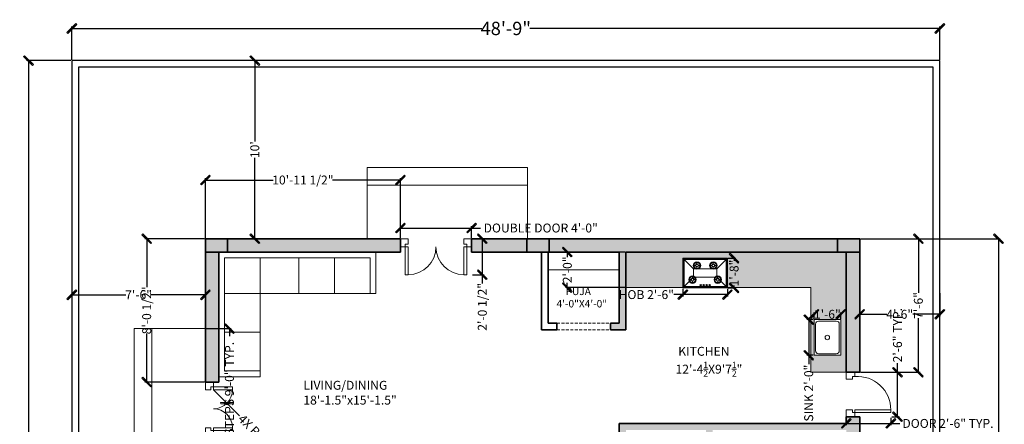
# Model space of a CAD drawing. Units: inches. Extents: x 1018 to 2596, y 723 to 1501.
# Tile 5 of 6: x 1018 to 1681, y 1229 to 1501. Entities that reach past the tile are written whole.
import ezdxf

# ---------------------------------------------------------------- set-up
doc = ezdxf.new("R2010")
doc.units = ezdxf.units.IN
doc.linetypes.add('DASHED2', pattern=[0.375, 0.25, -0.125])
doc.layers.get('Defpoints').update_dxf_attribs({"lineweight": 0})
for name, color, linetype, lineweight in [('A-ANNO-DIMS', 2, 'Continuous', 13), ('A-AREA-IDEN', 7, 'Continuous', 18), ('A-COLS', 7, 'Continuous', 35), ('A-DOOR', 4, 'Continuous', 18), ('A-EQPM', 8, 'Continuous', 18), ('A-FLOR-CASE', 8, 'Continuous', 18), ('A-FLOR-CASE-PATT', 9, 'Continuous', 9), ('A-FLOR-FIXT', 9, 'Continuous', 18), ('A-FLOR-STRS', 7, 'Continuous', 18), ('A-FURN', 8, 'Continuous', 13), ('A-WALL', 7, 'Continuous', 35), ('A-WALL-OVHD', 7, 'DASHED2', 13), ('C-PROP', 7, 'Continuous', 25)]:
    doc.layers.add(name, color=color, linetype=linetype, lineweight=lineweight)
doc.layers.add('A-WALL-PATT', color=9, linetype='Continuous', lineweight=9, true_color=0xc7c8ca)
doc.styles.get("Standard").update_dxf_attribs({"font": 'arial.ttf'})
doc.dimstyles.new('saketh', dxfattribs={"dimtxt": 6, "dimasz": 6, "dimexe": 1.25, "dimexo": 0.625, "dimtad": 0, "dimdec": 1, "dimlunit": 4, "dimtxsty": 'Standard', "dimblk": 'ARCHTICK', "dimcen": 2.5, "dimclrd": 256, "dimclre": 1, "dimadec": 0, "dimazin": 0, "dimtfac": 1, "dimtdec": 1, "dimtmove": 0, "dimatfit": 3, "dimldrblk": 'ARCHTICK', "dimfxl": 1, "dimtolj": 1, "dimarcsym": 0})

# ---------------------------------------------------------------- blocks, each defined once
blk = doc.blocks.new('4 feet double door')
at = {"layer": 'A-DOOR'}
for points in [[(3.28, 5.56), (3.28, 24.28), (5.25, 24.28), (5.25, 5.56)], [(44.72, 5.56), (44.72, 24.28), (42.75, 24.28), (42.75, 5.56)], [(3.28, 5.56), (0, 5.56), (0, 0), (5.25, 0), (5.25, 3.59), (3.28, 3.59)], [(44.72, 5.56), (48, 5.56), (48, 0), (42.75, 0), (42.75, 3.59), (44.72, 3.59)]]:
    blk.add_lwpolyline(points, close=True, dxfattribs=at)
at = {"layer": 'A-DOOR', "ltscale": 0.1}
for centre, start, end in [((5.25, 5.53), 0.09557, 90), ((42.75, 5.53), 90, 179.90443)]:
    blk.add_arc(centre, 18.75, start, end, dxfattribs=at)
blk = doc.blocks.new('3 1')
at = {"layer": 'A-DOOR'}
for points in [[(-32.72, 5.56), (-32.72, 18.28), (-30.75, 18.28), (-30.75, 5.56)], [(-3.28, 5.56), (-3.28, 18.28), (-5.25, 18.28), (-5.25, 5.56)], [(-32.72, 5.56), (-36, 5.56), (-36, 0), (-30.75, 0), (-30.75, 3.59), (-32.72, 3.59)], [(-5.25, 3.59), (-5.25, 0), (0, 0), (0, 5.56), (-3.28, 5.56), (-3.28, 3.59)]]:
    blk.add_lwpolyline(points, close=True, dxfattribs=at)
at = {"layer": 'A-DOOR', "ltscale": 0.1}
for centre, start, end in [((-30.75, 5.53), 0.1406, 90), ((-5.25, 5.53), 90, 179.8594)]:
    blk.add_arc(centre, 12.75, start, end, dxfattribs=at)
blk = doc.blocks.new('2 feet 6 inch door')
at = {"layer": 'A-DOOR'}
for points in [[(2.92, 5.83), (2.92, 30), (4.67, 30), (4.67, 5.83)], [(2.92, 4.08), (4.67, 4.08), (4.67, 0), (0, 0), (0, 5.83), (2.92, 5.83)], [(27.08, 5.83), (27.08, 4.08), (25.33, 4.08), (25.33, 0), (30, 0), (30, 5.83)]]:
    blk.add_lwpolyline(points, close=True, dxfattribs=at)
at = {"layer": 'A-DOOR', "ltscale": 0.1}
blk.add_arc((4.67, 7.52), 22.48, 355.69715, 90, dxfattribs=at)
blk = doc.blocks.new('_ArchTick')
for p, q in [((0.45, 0.55), (-0.55, -0.45)), ((-0.45, -0.55), (0.55, 0.45)), ((0.55, 0.45), (0.45, 0.55)), ((-0.55, -0.45), (-0.45, -0.55))]:
    blk.add_line(p, q)
mesh = blk.add_polyface()
corners = [(-0.45, -0.55), (0.45, 0.55), (-0.55, -0.45), (0.55, 0.45)]
mesh.append_faces([[corners[k] for k in face] for face in [(0, 1, 2), (1, 0, 3)]], dxfattribs={"vtx0": -1})
blk = doc.blocks.new('*D48')
at = {"layer": 'A-ANNO-DIMS', "color": 0, "lineweight": -2, "transparency": 16777216}
for p, q in [((1052.69, 1474.35), (1052.69, 1496.67)), ((1052.69, 1495.42), (1328.92, 1495.42)), ((1637.69, 1495.42), (1361.45, 1495.42)), ((1637.69, 1474.35), (1637.69, 1496.67))]:
    blk.add_line(p, q, dxfattribs=at)
at = {"layer": 'Defpoints', "color": 0, "transparency": 16777216}
for p in [(1637.69, 1495.42), (1052.69, 1473.73), (1637.69, 1473.73)]:
    blk.add_point(p, dxfattribs=at)
at = {"layer": 'A-ANNO-DIMS', "color": 0, "lineweight": -2, "transparency": 16777216, "xscale": 6, "yscale": 6, "zscale": 6, "rotation": 180}
blk.add_blockref('_ArchTick', (1052.69, 1495.42), dxfattribs=at)
at = {"layer": 'A-ANNO-DIMS', "color": 0, "lineweight": -2, "transparency": 16777216, "xscale": 6, "yscale": 6, "zscale": 6}
blk.add_blockref('_ArchTick', (1637.69, 1495.42), dxfattribs=at)
at = {"layer": 'A-ANNO-DIMS', "color": 0, "transparency": 16777216, "insert": (1345.19, 1495.42), "char_height": 9, "attachment_point": 5}
blk.add_mtext('\\A1;48\'-9"', dxfattribs=at)
blk = doc.blocks.new('*D49')
at = {"layer": 'A-ANNO-DIMS', "color": 0, "lineweight": -2, "transparency": 16777216}
for p, q in [((1052.06, 1473.73), (1022.21, 1473.73)), ((1023.46, 1473.73), (1023.46, 1116.33)), ((1023.46, 726.73), (1023.46, 1084.12)), ((1052.06, 726.73), (1022.21, 726.73))]:
    blk.add_line(p, q, dxfattribs=at)
at = {"layer": 'Defpoints', "color": 0, "transparency": 16777216}
for p in [(1052.69, 1473.73), (1023.46, 726.73), (1052.69, 726.73)]:
    blk.add_point(p, dxfattribs=at)
at = {"layer": 'A-ANNO-DIMS', "color": 0, "lineweight": -2, "transparency": 16777216, "xscale": 6, "yscale": 6, "zscale": 6}
for p, rotation in [((1023.46, 1473.73), 90), ((1023.46, 726.73), 270)]:
    blk.add_blockref('_ArchTick', p, dxfattribs=dict(at, rotation=rotation))
at = {"layer": 'A-ANNO-DIMS', "color": 0, "transparency": 16777216, "insert": (1023.46, 1100.23), "char_height": 9, "attachment_point": 5, "rotation": 90}
blk.add_mtext('\\A1;62\'-3"', dxfattribs=at)
blk = doc.blocks.new('*D50')
at = {"layer": 'A-ANNO-DIMS', "color": 0, "lineweight": -2, "transparency": 16777216}
for p, q in [((1052.69, 1321.53), (1052.69, 1314.64)), ((1142.69, 1321.53), (1142.69, 1314.64)), ((1052.69, 1315.89), (1089.11, 1315.89)), ((1142.69, 1315.89), (1106.26, 1315.89))]:
    blk.add_line(p, q, dxfattribs=at)
at = {"layer": 'Defpoints', "color": 0, "transparency": 16777216}
for p in [(1052.69, 1322.15), (1142.69, 1322.15), (1052.69, 1315.89)]:
    blk.add_point(p, dxfattribs=at)
at = {"layer": 'A-ANNO-DIMS', "color": 0, "lineweight": -2, "transparency": 16777216, "xscale": 6, "yscale": 6, "zscale": 6, "rotation": 180}
blk.add_blockref('_ArchTick', (1052.69, 1315.89), dxfattribs=at)
at = {"layer": 'A-ANNO-DIMS', "color": 0, "lineweight": -2, "transparency": 16777216, "xscale": 6, "yscale": 6, "zscale": 6}
blk.add_blockref('_ArchTick', (1142.69, 1315.89), dxfattribs=at)
at = {"layer": 'A-ANNO-DIMS', "color": 0, "transparency": 16777216, "insert": (1097.69, 1315.89), "char_height": 6, "attachment_point": 5}
blk.add_mtext('\\A1;7\'-6"', dxfattribs=at)
blk = doc.blocks.new('*D51')
at = {"layer": 'A-ANNO-DIMS', "color": 0, "lineweight": -2, "transparency": 16777216}
for p, q in [((1182.33, 1473.73), (1174.76, 1473.73)), ((1176.01, 1473.73), (1176.01, 1419.16)), ((1176.01, 1353.73), (1176.01, 1408.29)), ((1182.33, 1353.73), (1174.76, 1353.73))]:
    blk.add_line(p, q, dxfattribs=at)
at = {"layer": 'Defpoints', "color": 0, "transparency": 16777216}
for p in [(1176.01, 1473.73), (1182.95, 1473.73), (1182.95, 1353.73)]:
    blk.add_point(p, dxfattribs=at)
at = {"layer": 'A-ANNO-DIMS', "color": 0, "lineweight": -2, "transparency": 16777216, "xscale": 6, "yscale": 6, "zscale": 6}
for p, rotation in [((1176.01, 1473.73), 90), ((1176.01, 1353.73), 270)]:
    blk.add_blockref('_ArchTick', p, dxfattribs=dict(at, rotation=rotation))
at = {"layer": 'A-ANNO-DIMS', "color": 0, "transparency": 16777216, "insert": (1176.01, 1413.73), "char_height": 6, "attachment_point": 5, "rotation": 90}
blk.add_mtext("\\A1;10'", dxfattribs=at)
blk = doc.blocks.new('*D52')
at = {"layer": 'A-ANNO-DIMS', "color": 0, "lineweight": -2, "transparency": 16777216}
for p, q in [((1583.69, 1316.96), (1583.69, 1301.54)), ((1637.69, 1316.96), (1637.69, 1301.54)), ((1583.69, 1302.79), (1601.97, 1302.79)), ((1637.69, 1302.79), (1619.41, 1302.79))]:
    blk.add_line(p, q, dxfattribs=at)
at = {"layer": 'Defpoints', "color": 0, "transparency": 16777216}
for p in [(1583.69, 1317.58), (1637.69, 1317.58), (1637.69, 1302.79)]:
    blk.add_point(p, dxfattribs=at)
at = {"layer": 'A-ANNO-DIMS', "color": 0, "lineweight": -2, "transparency": 16777216, "xscale": 6, "yscale": 6, "zscale": 6, "rotation": 180}
blk.add_blockref('_ArchTick', (1583.69, 1302.79), dxfattribs=at)
at = {"layer": 'A-ANNO-DIMS', "color": 0, "lineweight": -2, "transparency": 16777216, "xscale": 6, "yscale": 6, "zscale": 6}
blk.add_blockref('_ArchTick', (1637.69, 1302.79), dxfattribs=at)
at = {"layer": 'A-ANNO-DIMS', "color": 0, "transparency": 16777216, "insert": (1610.69, 1302.79), "char_height": 6, "attachment_point": 5}
blk.add_mtext('\\A1;4\'-6"', dxfattribs=at)
blk = doc.blocks.new('CHIMNEYU')
at = {"layer": 'A-FURN', "ltscale": 2.5}
for p, q in [((-25.3, 14.2), (-33.3, 22.2)), ((-7.8, 14.2), (0.2, 22.2)), ((-25.3, 7.8), (-33.3, -0.2)), ((-7.8, 7.8), (0.2, -0.2))]:
    blk.add_line(p, q, dxfattribs=at)
for points in [[(-33.3, -0.2), (0.2, -0.2), (0.2, 22.2), (-33.3, 22.2)], [(-33.1, 0), (0, 0), (0, 22), (-33.1, 22)], [(-32.3, 0.8), (-0.8, 0.8), (-0.8, 21.2), (-32.3, 21.2)], [(-25.3, 7.8), (-7.8, 7.8), (-7.8, 14.2), (-25.3, 14.2)]]:
    blk.add_lwpolyline(points, close=True, dxfattribs=at)
blk = doc.blocks.new('stove')
at = {"layer": 'A-FURN'}
for p, q in [((4.46, 14.48), (5.96, 14.48)), ((6.5, 16.48), (6.5, 14.98)), ((6.5, 12.48), (6.5, 13.98)), ((8.46, 14.48), (6.96, 14.48)), ((21.46, 14.48), (22.96, 14.48)), ((23.5, 16.48), (23.5, 14.98)), ((23.5, 12.48), (23.5, 13.98)), ((25.46, 14.48), (23.96, 14.48)), ((9.5, 6.93), (9.5, 5.43)), ((20.5, 6.93), (20.5, 5.43)), ((7.46, 4.93), (8.96, 4.93)), ((9.5, 2.93), (9.5, 4.43)), ((11.46, 4.93), (9.96, 4.93)), ((18.46, 4.93), (19.96, 4.93)), ((20.5, 2.93), (20.5, 4.43)), ((22.46, 4.93), (20.96, 4.93))]:
    blk.add_line(p, q, dxfattribs=at)
for centre, radius in [((6.5, 14.48), 2.5), ((6.5, 14.48), 2), ((6.5, 14.48), 1), ((12, 18.23), 0.5), ((14, 18.23), 0.5), ((16, 18.23), 0.5), ((18, 18.23), 0.5), ((23.5, 14.48), 2.5), ((23.5, 14.48), 2), ((23.5, 14.48), 1), ((9.5, 4.93), 2.5), ((9.5, 4.93), 2), ((20.5, 4.93), 2.5), ((20.5, 4.93), 2), ((9.5, 4.93), 1), ((20.5, 4.93), 1)]:
    blk.add_circle(centre, radius, dxfattribs=at)
at = {"layer": 'A-FURN', "xscale": 0.8955224042543976, "yscale": 0.8955224042543976, "zscale": 0.8955224042543976}
blk.add_blockref('CHIMNEYU', (29.82, 0.18), dxfattribs=at)
blk = doc.blocks.new('sink')
at = {"layer": 'A-FURN'}
for p, q in [((-9, 12), (9, 12)), ((-9, -12), (-9, 12)), ((-8, -9), (-8, 9)), ((-6, 11), (6, 11)), ((8, 9), (8, -9)), ((9, 12), (9, -12)), ((9, -12), (-9, -12)), ((6, -11), (-6, -11))]:
    blk.add_line(p, q, dxfattribs=at)
blk.add_circle((0, 0), 1.53, dxfattribs=at)
for centre, start, end in [((-6, 9), 90, 180), ((6, 9), 0, 90), ((-6, -9), 180, 270), ((6, -9), 270, 0)]:
    blk.add_arc(centre, 2, start, end, dxfattribs=at)
blk = doc.blocks.new('COLUMN-15X9-IN')
h = blk.add_hatch(color=256)
h.dxf.hatch_style = 1
h.paths.add_polyline_path([(15, 0), (15, 9), (0, 9), (0, 0)])
blk.add_lwpolyline([(15, 9), (15, 0), (0, 0), (0, 9)], close=True)
blk = doc.blocks.new('ENTRY-STEP-108X48-IN')
for p, q in [((0, 0), (0, 108)), ((0, 108), (12, 108)), ((12, 0), (12, 108)), ((48, 108), (12, 108)), ((0, 0), (12, 0)), ((48, 0), (12, 0))]:
    blk.add_line(p, q)
blk = doc.blocks.new('*D61')
at = {"layer": 'A-ANNO-DIMS', "color": 1, "lineweight": -2, "transparency": 16777216}
for p, q in [((1574.69, 1233.1), (1574.69, 1227.98)), ((1604.69, 1233.1), (1604.69, 1227.98))]:
    blk.add_line(p, q, dxfattribs=at)
at = {"layer": 'A-ANNO-DIMS', "lineweight": -2, "transparency": 16777216}
for p, q in [((1574.69, 1229.23), (1604.69, 1229.23)), ((1604.69, 1229.23), (1610.69, 1229.23))]:
    blk.add_line(p, q, dxfattribs=at)
at = {"layer": 'Defpoints', "color": 0, "transparency": 16777216}
for p in [(1574.69, 1233.73), (1604.69, 1233.73), (1604.69, 1229.23)]:
    blk.add_point(p, dxfattribs=at)
at = {"layer": 'A-ANNO-DIMS', "lineweight": -2, "transparency": 16777216, "xscale": 6, "yscale": 6, "zscale": 6, "rotation": 180}
blk.add_blockref('_ArchTick', (1574.69, 1229.23), dxfattribs=at)
at = {"layer": 'A-ANNO-DIMS', "lineweight": -2, "transparency": 16777216, "xscale": 6, "yscale": 6, "zscale": 6}
blk.add_blockref('_ArchTick', (1604.69, 1229.23), dxfattribs=at)
at = {"layer": 'A-ANNO-DIMS', "color": 0, "transparency": 16777216, "insert": (1643.19, 1229.23), "char_height": 6, "attachment_point": 5}
blk.add_mtext('\\A1;DOOR 2\'-6" TYP.', dxfattribs=at)
blk = doc.blocks.new('*D62')
at = {"layer": 'A-ANNO-DIMS', "lineweight": -2, "transparency": 16777216}
for p, q in [((1609.19, 1263.73), (1609.19, 1269.73)), ((1609.19, 1233.73), (1609.19, 1263.73))]:
    blk.add_line(p, q, dxfattribs=at)
at = {"layer": 'A-ANNO-DIMS', "color": 1, "lineweight": -2, "transparency": 16777216}
for p, q in [((1605.31, 1263.73), (1610.44, 1263.73)), ((1605.31, 1233.73), (1610.44, 1233.73))]:
    blk.add_line(p, q, dxfattribs=at)
at = {"layer": 'Defpoints', "color": 0, "transparency": 16777216}
for p in [(1604.69, 1263.73), (1609.19, 1263.73), (1604.69, 1233.73)]:
    blk.add_point(p, dxfattribs=at)
at = {"layer": 'A-ANNO-DIMS', "lineweight": -2, "transparency": 16777216, "xscale": 6, "yscale": 6, "zscale": 6}
for p, rotation in [((1609.19, 1263.73), 90), ((1609.19, 1233.73), 270)]:
    blk.add_blockref('_ArchTick', p, dxfattribs=dict(at, rotation=rotation))
at = {"layer": 'A-ANNO-DIMS', "color": 0, "transparency": 16777216, "insert": (1609.19, 1288.69), "char_height": 6, "attachment_point": 5, "rotation": 90}
blk.add_mtext('\\A1;2\'-6" TYP.', dxfattribs=at)
blk = doc.blocks.new('*D69')
at = {"layer": 'A-ANNO-DIMS', "color": 1, "lineweight": -2, "transparency": 16777216}
for p, q in [((1143.31, 1293.11), (1160.14, 1293.11)), ((1143.31, 1185.11), (1160.14, 1185.11))]:
    blk.add_line(p, q, dxfattribs=at)
at = {"layer": 'A-ANNO-DIMS', "lineweight": -2, "transparency": 16777216}
for p, q in [((1158.89, 1293.11), (1158.89, 1288.14)), ((1158.89, 1185.11), (1158.89, 1190.09))]:
    blk.add_line(p, q, dxfattribs=at)
at = {"layer": 'Defpoints', "color": 0, "transparency": 16777216}
for p in [(1142.69, 1293.11), (1158.89, 1293.11), (1142.69, 1185.11)]:
    blk.add_point(p, dxfattribs=at)
at = {"layer": 'A-ANNO-DIMS', "lineweight": -2, "transparency": 16777216, "xscale": 6, "yscale": 6, "zscale": 6}
for p, rotation in [((1158.89, 1293.11), 90), ((1158.89, 1185.11), 270)]:
    blk.add_blockref('_ArchTick', p, dxfattribs=dict(at, rotation=rotation))
at = {"layer": 'A-ANNO-DIMS', "color": 0, "transparency": 16777216, "insert": (1158.89, 1239.11), "char_height": 6, "attachment_point": 5, "rotation": 90}
blk.add_mtext('\\A1;ENTRY STEPS 9\'-0" TYP.', dxfattribs=at)
blk = doc.blocks.new('*D71')
at = {"layer": 'A-ANNO-DIMS', "color": 1, "lineweight": -2, "transparency": 16777216}
for p, q in [((1274.14, 1354.35), (1274.14, 1362.18)), ((1322.14, 1354.35), (1322.14, 1362.18))]:
    blk.add_line(p, q, dxfattribs=at)
at = {"layer": 'A-ANNO-DIMS', "lineweight": -2, "transparency": 16777216}
for p, q in [((1274.14, 1360.93), (1322.14, 1360.93)), ((1322.14, 1360.93), (1328.14, 1360.93))]:
    blk.add_line(p, q, dxfattribs=at)
at = {"layer": 'Defpoints', "color": 0, "transparency": 16777216}
for p in [(1322.14, 1360.93), (1274.14, 1353.73), (1322.14, 1353.73)]:
    blk.add_point(p, dxfattribs=at)
at = {"layer": 'A-ANNO-DIMS', "lineweight": -2, "transparency": 16777216, "xscale": 6, "yscale": 6, "zscale": 6, "rotation": 180}
blk.add_blockref('_ArchTick', (1274.14, 1360.93), dxfattribs=at)
at = {"layer": 'A-ANNO-DIMS', "lineweight": -2, "transparency": 16777216, "xscale": 6, "yscale": 6, "zscale": 6}
blk.add_blockref('_ArchTick', (1322.14, 1360.93), dxfattribs=at)
at = {"layer": 'A-ANNO-DIMS', "color": 0, "transparency": 16777216, "insert": (1368.72, 1360.93), "char_height": 6, "attachment_point": 5}
blk.add_mtext('\\A1;DOUBLE DOOR 4\'-0"', dxfattribs=at)
blk = doc.blocks.new('*D72')
at = {"layer": 'A-ANNO-DIMS', "color": 1, "lineweight": -2, "transparency": 16777216}
for p, q in [((1322.76, 1353.73), (1330.59, 1353.73)), ((1322.76, 1329.44), (1330.59, 1329.44))]:
    blk.add_line(p, q, dxfattribs=at)
at = {"layer": 'A-ANNO-DIMS', "lineweight": -2, "transparency": 16777216}
for p, q in [((1329.34, 1353.73), (1329.34, 1329.44)), ((1329.34, 1329.44), (1329.34, 1323.44))]:
    blk.add_line(p, q, dxfattribs=at)
at = {"layer": 'Defpoints', "color": 0, "transparency": 16777216}
for p in [(1322.14, 1353.73), (1322.14, 1329.44), (1329.34, 1329.44)]:
    blk.add_point(p, dxfattribs=at)
at = {"layer": 'A-ANNO-DIMS', "lineweight": -2, "transparency": 16777216, "xscale": 6, "yscale": 6, "zscale": 6}
for p, rotation in [((1329.34, 1353.73), 90), ((1329.34, 1329.44), 270)]:
    blk.add_blockref('_ArchTick', p, dxfattribs=dict(at, rotation=rotation))
at = {"layer": 'A-ANNO-DIMS', "color": 0, "transparency": 16777216, "insert": (1329.34, 1307.8), "char_height": 6, "attachment_point": 5, "rotation": 90}
blk.add_mtext('\\A1;2\'-0 1/2"', dxfattribs=at)
blk = doc.blocks.new('*D73')
at = {"layer": 'A-ANNO-DIMS', "lineweight": -2, "transparency": 16777216}
for p, q in [((1464.54, 1316.05), (1458.54, 1316.05)), ((1494.54, 1316.05), (1464.54, 1316.05))]:
    blk.add_line(p, q, dxfattribs=at)
at = {"layer": 'A-ANNO-DIMS', "color": 1, "lineweight": -2, "transparency": 16777216}
for p, q in [((1464.54, 1319.92), (1464.54, 1314.8)), ((1494.54, 1319.92), (1494.54, 1314.8))]:
    blk.add_line(p, q, dxfattribs=at)
at = {"layer": 'Defpoints', "color": 0, "transparency": 16777216}
for p in [(1464.54, 1320.55), (1464.54, 1316.05), (1494.54, 1320.55)]:
    blk.add_point(p, dxfattribs=at)
at = {"layer": 'A-ANNO-DIMS', "lineweight": -2, "transparency": 16777216, "xscale": 6, "yscale": 6, "zscale": 6, "rotation": 180}
blk.add_blockref('_ArchTick', (1464.54, 1316.05), dxfattribs=at)
at = {"layer": 'A-ANNO-DIMS', "lineweight": -2, "transparency": 16777216, "xscale": 6, "yscale": 6, "zscale": 6}
blk.add_blockref('_ArchTick', (1494.54, 1316.05), dxfattribs=at)
at = {"layer": 'A-ANNO-DIMS', "color": 0, "transparency": 16777216, "insert": (1439.86, 1316.05), "char_height": 6, "attachment_point": 5}
blk.add_mtext('\\A1;HOB 2\'-6"', dxfattribs=at)
blk = doc.blocks.new('*D74')
at = {"layer": 'A-ANNO-DIMS', "color": 1, "lineweight": -2, "transparency": 16777216}
for p, q in [((1495.17, 1340.61), (1500.29, 1340.61)), ((1495.17, 1320.55), (1500.29, 1320.55))]:
    blk.add_line(p, q, dxfattribs=at)
at = {"layer": 'A-ANNO-DIMS', "lineweight": -2, "transparency": 16777216}
for p, q in [((1499.04, 1340.61), (1499.04, 1338.89)), ((1499.04, 1320.55), (1499.04, 1322.26))]:
    blk.add_line(p, q, dxfattribs=at)
at = {"layer": 'Defpoints', "color": 0, "transparency": 16777216}
for p in [(1494.54, 1340.61), (1494.54, 1320.55), (1499.04, 1320.55)]:
    blk.add_point(p, dxfattribs=at)
at = {"layer": 'A-ANNO-DIMS', "lineweight": -2, "transparency": 16777216, "xscale": 6, "yscale": 6, "zscale": 6}
for p, rotation in [((1499.04, 1340.61), 90), ((1499.04, 1320.55), 270)]:
    blk.add_blockref('_ArchTick', p, dxfattribs=dict(at, rotation=rotation))
at = {"layer": 'A-ANNO-DIMS', "color": 0, "transparency": 16777216, "insert": (1499.04, 1330.58), "char_height": 6, "attachment_point": 5, "rotation": 90}
blk.add_mtext('\\A1;1\'-8"', dxfattribs=at)
blk = doc.blocks.new('*D75')
at = {"layer": 'A-ANNO-DIMS', "color": 1, "lineweight": -2, "transparency": 16777216}
for p, q in [((1552.3, 1299.18), (1548.08, 1299.18)), ((1552.3, 1275.18), (1548.08, 1275.18))]:
    blk.add_line(p, q, dxfattribs=at)
at = {"layer": 'A-ANNO-DIMS', "lineweight": -2, "transparency": 16777216}
for p, q in [((1549.33, 1299.18), (1549.33, 1275.18)), ((1549.33, 1275.18), (1549.33, 1269.18))]:
    blk.add_line(p, q, dxfattribs=at)
at = {"layer": 'Defpoints', "color": 0, "transparency": 16777216}
for p in [(1552.93, 1299.18), (1549.33, 1275.18), (1552.93, 1275.18)]:
    blk.add_point(p, dxfattribs=at)
at = {"layer": 'A-ANNO-DIMS', "lineweight": -2, "transparency": 16777216, "xscale": 6, "yscale": 6, "zscale": 6}
for p, rotation in [((1549.33, 1299.18), 90), ((1549.33, 1275.18), 270)]:
    blk.add_blockref('_ArchTick', p, dxfattribs=dict(at, rotation=rotation))
at = {"layer": 'A-ANNO-DIMS', "color": 0, "transparency": 16777216, "insert": (1549.33, 1249.64), "char_height": 6, "attachment_point": 5, "rotation": 90}
blk.add_mtext('\\A1;SINK 2\'-0"', dxfattribs=at)
blk = doc.blocks.new('*D76')
at = {"layer": 'A-ANNO-DIMS', "color": 1, "lineweight": -2, "transparency": 16777216}
for p, q in [((1552.93, 1299.8), (1552.93, 1304.03)), ((1570.93, 1299.8), (1570.93, 1304.03))]:
    blk.add_line(p, q, dxfattribs=at)
at = {"layer": 'A-ANNO-DIMS', "lineweight": -2, "transparency": 16777216}
for p, q in [((1552.93, 1302.78), (1553.61, 1302.78)), ((1570.93, 1302.78), (1570.25, 1302.78))]:
    blk.add_line(p, q, dxfattribs=at)
at = {"layer": 'Defpoints', "color": 0, "transparency": 16777216}
for p in [(1552.93, 1302.78), (1552.93, 1299.18), (1570.93, 1299.18)]:
    blk.add_point(p, dxfattribs=at)
at = {"layer": 'A-ANNO-DIMS', "lineweight": -2, "transparency": 16777216, "xscale": 6, "yscale": 6, "zscale": 6, "rotation": 180}
blk.add_blockref('_ArchTick', (1552.93, 1302.78), dxfattribs=at)
at = {"layer": 'A-ANNO-DIMS', "lineweight": -2, "transparency": 16777216, "xscale": 6, "yscale": 6, "zscale": 6}
blk.add_blockref('_ArchTick', (1570.93, 1302.78), dxfattribs=at)
at = {"layer": 'A-ANNO-DIMS', "color": 0, "transparency": 16777216, "insert": (1561.93, 1302.78), "char_height": 6, "attachment_point": 5}
blk.add_mtext('\\A1;1\'-6"', dxfattribs=at)
blk = doc.blocks.new('*D77')
at = {"layer": 'A-ANNO-DIMS', "color": 1, "lineweight": -2, "transparency": 16777216}
for p, q in [((1514.73, 1215.58), (1514.73, 1219.12)), ((1534.19, 1215.58), (1534.19, 1219.12))]:
    blk.add_line(p, q, dxfattribs=at)
at = {"layer": 'A-ANNO-DIMS', "lineweight": -2, "transparency": 16777216}
for p, q in [((1514.73, 1217.87), (1534.19, 1217.87)), ((1534.19, 1217.87), (1540.19, 1217.87))]:
    blk.add_line(p, q, dxfattribs=at)
at = {"layer": 'Defpoints', "color": 0, "transparency": 16777216}
for p in [(1514.73, 1214.95), (1534.19, 1217.87), (1534.19, 1214.95)]:
    blk.add_point(p, dxfattribs=at)
at = {"layer": 'A-ANNO-DIMS', "lineweight": -2, "transparency": 16777216, "xscale": 6, "yscale": 6, "zscale": 6, "rotation": 180}
blk.add_blockref('_ArchTick', (1514.73, 1217.87), dxfattribs=at)
at = {"layer": 'A-ANNO-DIMS', "lineweight": -2, "transparency": 16777216, "xscale": 6, "yscale": 6, "zscale": 6}
blk.add_blockref('_ArchTick', (1534.19, 1217.87), dxfattribs=at)
at = {"layer": 'A-ANNO-DIMS', "color": 0, "transparency": 16777216, "insert": (1564.05, 1217.87), "char_height": 6, "attachment_point": 5}
blk.add_mtext('\\A1;WC 1\'-7 1/2"', dxfattribs=at)
blk = doc.blocks.new('*D80')
at = {"layer": 'A-ANNO-DIMS', "color": 1, "lineweight": -2, "transparency": 16777216}
for p, q in [((1584.31, 1353.73), (1678.49, 1353.73)), ((1584.31, 993.73), (1678.49, 993.73))]:
    blk.add_line(p, q, dxfattribs=at)
at = {"layer": 'A-ANNO-DIMS', "lineweight": -2, "transparency": 16777216}
for p, q in [((1677.24, 1353.73), (1677.24, 1184.65)), ((1677.24, 993.73), (1677.24, 1162.8))]:
    blk.add_line(p, q, dxfattribs=at)
at = {"layer": 'Defpoints', "color": 0, "transparency": 16777216}
for p in [(1583.69, 1353.73), (1677.24, 1353.73), (1583.69, 993.73)]:
    blk.add_point(p, dxfattribs=at)
at = {"layer": 'A-ANNO-DIMS', "lineweight": -2, "transparency": 16777216, "xscale": 6, "yscale": 6, "zscale": 6}
for p, rotation in [((1677.24, 1353.73), 90), ((1677.24, 993.73), 270)]:
    blk.add_blockref('_ArchTick', p, dxfattribs=dict(at, rotation=rotation))
at = {"layer": 'A-ANNO-DIMS', "color": 0, "transparency": 16777216, "insert": (1677.24, 1173.73), "char_height": 6, "attachment_point": 5, "rotation": 90}
blk.add_mtext('\\A1;30\'-0"', dxfattribs=at)
blk = doc.blocks.new('*D91')
at = {"layer": 'A-ANNO-DIMS', "color": 1, "lineweight": -2, "transparency": 16777216}
for p, q in [((1142.69, 1354.35), (1142.69, 1394.53)), ((1274.14, 1354.35), (1274.14, 1394.53))]:
    blk.add_line(p, q, dxfattribs=at)
at = {"layer": 'A-ANNO-DIMS', "lineweight": -2, "transparency": 16777216}
for p, q in [((1142.69, 1393.28), (1188.44, 1393.28)), ((1274.14, 1393.28), (1228.38, 1393.28))]:
    blk.add_line(p, q, dxfattribs=at)
at = {"layer": 'Defpoints', "color": 0, "transparency": 16777216}
for p in [(1274.14, 1393.28), (1142.69, 1353.73), (1274.14, 1353.73)]:
    blk.add_point(p, dxfattribs=at)
at = {"layer": 'A-ANNO-DIMS', "lineweight": -2, "transparency": 16777216, "xscale": 6, "yscale": 6, "zscale": 6, "rotation": 180}
blk.add_blockref('_ArchTick', (1142.69, 1393.28), dxfattribs=at)
at = {"layer": 'A-ANNO-DIMS', "lineweight": -2, "transparency": 16777216, "xscale": 6, "yscale": 6, "zscale": 6}
blk.add_blockref('_ArchTick', (1274.14, 1393.28), dxfattribs=at)
at = {"layer": 'A-ANNO-DIMS', "color": 0, "transparency": 16777216, "insert": (1208.41, 1393.28), "char_height": 6, "attachment_point": 5}
blk.add_mtext('\\A1;10\'-11 1/2"', dxfattribs=at)
blk = doc.blocks.new('*D92')
at = {"layer": 'A-ANNO-DIMS', "color": 1, "lineweight": -2, "transparency": 16777216}
for p, q in [((1142.06, 1353.73), (1101.89, 1353.73)), ((1142.06, 1257.11), (1101.89, 1257.11))]:
    blk.add_line(p, q, dxfattribs=at)
at = {"layer": 'A-ANNO-DIMS', "lineweight": -2, "transparency": 16777216}
for p, q in [((1103.14, 1353.73), (1103.14, 1321.01)), ((1103.14, 1257.11), (1103.14, 1289.83))]:
    blk.add_line(p, q, dxfattribs=at)
at = {"layer": 'Defpoints', "color": 0, "transparency": 16777216}
for p in [(1103.14, 1353.73), (1142.69, 1353.73), (1142.69, 1257.11)]:
    blk.add_point(p, dxfattribs=at)
at = {"layer": 'A-ANNO-DIMS', "lineweight": -2, "transparency": 16777216, "xscale": 6, "yscale": 6, "zscale": 6}
for p, rotation in [((1103.14, 1353.73), 90), ((1103.14, 1257.11), 270)]:
    blk.add_blockref('_ArchTick', p, dxfattribs=dict(at, rotation=rotation))
at = {"layer": 'A-ANNO-DIMS', "color": 0, "transparency": 16777216, "insert": (1103.14, 1305.42), "char_height": 6, "attachment_point": 5, "rotation": 90}
blk.add_mtext('\\A1;8\'-0 1/2"', dxfattribs=at)
blk = doc.blocks.new('*D95')
at = {"layer": 'A-ANNO-DIMS', "color": 1, "lineweight": -2, "transparency": 16777216}
for p, q in [((1584.31, 1353.73), (1624.49, 1353.73)), ((1584.31, 1263.73), (1624.49, 1263.73))]:
    blk.add_line(p, q, dxfattribs=at)
at = {"layer": 'A-ANNO-DIMS', "lineweight": -2, "transparency": 16777216}
for p, q in [((1623.24, 1353.73), (1623.24, 1317.3)), ((1623.24, 1263.73), (1623.24, 1300.15))]:
    blk.add_line(p, q, dxfattribs=at)
at = {"layer": 'Defpoints', "color": 0, "transparency": 16777216}
for p in [(1583.69, 1353.73), (1583.69, 1263.73), (1623.24, 1263.73)]:
    blk.add_point(p, dxfattribs=at)
at = {"layer": 'A-ANNO-DIMS', "lineweight": -2, "transparency": 16777216, "xscale": 6, "yscale": 6, "zscale": 6}
for p, rotation in [((1623.24, 1353.73), 90), ((1623.24, 1263.73), 270)]:
    blk.add_blockref('_ArchTick', p, dxfattribs=dict(at, rotation=rotation))
at = {"layer": 'A-ANNO-DIMS', "color": 0, "transparency": 16777216, "insert": (1623.24, 1308.73), "char_height": 6, "attachment_point": 5, "rotation": 90}
blk.add_mtext('\\A1;7\'-6"', dxfattribs=at)
blk = doc.blocks.new('*D96')
at = {"layer": 'A-ANNO-DIMS', "color": 1, "lineweight": -2, "transparency": 16777216}
for p, q in [((1425.56, 1344.73), (1385.39, 1344.73)), ((1425.56, 1320.73), (1385.39, 1320.73))]:
    blk.add_line(p, q, dxfattribs=at)
at = {"layer": 'A-ANNO-DIMS', "lineweight": -2, "transparency": 16777216}
for p, q in [((1386.64, 1344.73), (1386.64, 1341.38)), ((1386.64, 1320.73), (1386.64, 1324.07))]:
    blk.add_line(p, q, dxfattribs=at)
at = {"layer": 'Defpoints', "color": 0, "transparency": 16777216}
for p in [(1386.64, 1344.73), (1426.19, 1344.73), (1426.19, 1320.73)]:
    blk.add_point(p, dxfattribs=at)
at = {"layer": 'A-ANNO-DIMS', "lineweight": -2, "transparency": 16777216, "xscale": 6, "yscale": 6, "zscale": 6}
for p, rotation in [((1386.64, 1344.73), 90), ((1386.64, 1320.73), 270)]:
    blk.add_blockref('_ArchTick', p, dxfattribs=dict(at, rotation=rotation))
at = {"layer": 'A-ANNO-DIMS', "color": 0, "transparency": 16777216, "insert": (1386.64, 1332.73), "char_height": 6, "attachment_point": 5, "rotation": 90}
blk.add_mtext('\\A1;2\'-0"', dxfattribs=at)
blk = doc.blocks.new('*D117')
at = {"layer": 'A-ANNO-DIMS', "lineweight": -2, "transparency": 16777216}
for p in [(1148.22, 1251.86), (1165.74, 1234.39)]:
    blk.add_line(p, (1157.25, 1242.86), dxfattribs=at)
at = {"layer": 'Defpoints', "color": 0, "transparency": 16777216}
for p in [(1148.22, 1251.86), (1157.25, 1242.86)]:
    blk.add_point(p, dxfattribs=at)
at = {"layer": 'A-ANNO-DIMS', "lineweight": -2, "transparency": 16777216, "xscale": 6, "yscale": 6, "zscale": 6, "rotation": 135.0720928995186}
blk.add_blockref('_ArchTick', (1157.25, 1242.86), dxfattribs=at)
at = {"layer": 'A-ANNO-DIMS', "color": 0, "transparency": 16777216, "insert": (1178.51, 1221.65), "char_height": 6, "attachment_point": 5, "rotation": 315.07209}
blk.add_mtext('\\A1;4X R1\'-1"', dxfattribs=at)

msp = doc.modelspace()

# ---------------------------------------------------------------- hatches: boundary and pattern name
at = {"layer": 'A-FLOR-CASE-PATT', "transparency": 33554531}
h = msp.add_hatch(color=256, dxfattribs=at)
h.dxf.hatch_style = 1
h.paths.add_polyline_path([(1550.69, 1320.73), (1550.69, 1263.73), (1574.69, 1263.73), (1574.69, 1344.73), (1568.69, 1344.73), (1426.19, 1344.73), (1426.19, 1320.73), (1464.54, 1320.73), (1464.54, 1340.61), (1494.54, 1340.61), (1494.54, 1320.73)])
h.paths.add_polyline_path([(1552.93, 1299.18), (1570.93, 1299.18), (1570.93, 1275.18), (1552.93, 1275.18)], flags=16)
h.paths.add_polyline_path([(1555.93, 1298.18), (1567.93, 1298.18, -0.414214), (1569.93, 1296.18), (1569.93, 1278.18, -0.414214), (1567.93, 1276.18), (1555.93, 1276.18, -0.414214), (1553.93, 1278.18), (1553.93, 1296.18, -0.414214)], flags=0)
h.paths.add_polyline_path([(1563.46, 1287.18, -1), (1560.4, 1287.18, -1)], flags=0)
at = {"layer": 'A-WALL-PATT', "transparency": 33554539}
h = msp.add_hatch(color=256, dxfattribs=at)
h.dxf.hatch_style = 1
h.paths.add_polyline_path([(1359.46, 1344.73), (1359.46, 1353.73), (1322.14, 1353.73), (1322.14, 1348.16), (1322.14, 1344.73)])
h.paths.add_polyline_path([(1374.46, 1353.73), (1374.46, 1344.73), (1421.69, 1344.73), (1421.69, 1296.73), (1415.69, 1296.73), (1415.69, 1292.23), (1426.19, 1292.23), (1426.19, 1344.73), (1568.69, 1344.73), (1568.69, 1353.73)])
h.paths.add_polyline_path([(1257.69, 1344.73), (1274.14, 1344.73), (1274.14, 1353.73), (1157.69, 1353.73), (1157.69, 1344.73)])
h.paths.add_polyline_path([(1151.69, 1344.73), (1142.69, 1344.73), (1142.69, 1257.11), (1148.25, 1257.11), (1151.69, 1257.11)])
h.paths.add_polyline_path([(1142.69, 1163.23), (1151.69, 1163.23), (1151.69, 1221.11), (1142.69, 1221.11)])
h.paths.add_polyline_path([(1151.69, 1154.23), (1142.69, 1154.23), (1142.69, 993.73), (1219.19, 993.73), (1219.19, 999.29), (1219.19, 1002.73), (1151.69, 1002.73)])
h.paths.add_polyline_path([(1327.94, 993.73), (1327.94, 1002.73), (1277.69, 1002.73), (1277.69, 1158.73), (1283.22, 1158.73), (1283.22, 1163.23), (1273.19, 1163.23), (1268.69, 1163.23), (1268.69, 1158.73), (1273.19, 1158.73), (1273.19, 1002.73), (1255.19, 1002.73), (1255.19, 993.73)])
h.paths.add_polyline_path([(1426.19, 1002.73), (1426.19, 1178.23), (1421.69, 1178.23), (1421.69, 1163.23), (1374.46, 1163.23), (1374.46, 1158.73), (1421.69, 1158.73), (1421.69, 1002.73), (1375.94, 1002.73), (1375.94, 993.73), (1478.69, 993.73), (1478.69, 1002.73)])
h.paths.add_polyline_path([(1583.69, 1233.73), (1574.69, 1233.73), (1574.69, 1229.23), (1421.69, 1229.23), (1421.69, 1220.23), (1426.19, 1220.23), (1426.19, 1224.73), (1480.19, 1224.73), (1480.19, 1158.73), (1489.19, 1158.73), (1489.19, 1163.23), (1484.69, 1163.23), (1484.69, 1224.73), (1508.69, 1224.73), (1574.69, 1224.73), (1574.69, 1163.23), (1583.69, 1163.23)])
h.paths.add_polyline_path([(1574.69, 1263.73), (1580.52, 1263.73), (1583.69, 1263.73), (1583.69, 1344.73), (1574.69, 1344.73)])
h.paths.add_polyline_path([(1583.69, 1154.23), (1574.69, 1154.23), (1574.69, 1002.73), (1583.69, 1002.73)])
h.paths.add_polyline_path([(1568.69, 993.73), (1568.69, 1002.73), (1526.69, 1002.73), (1526.69, 993.73)])
h.paths.add_polyline_path([(1359.46, 1158.73), (1359.46, 1163.23), (1325.22, 1163.23), (1325.22, 1158.73)])
h.paths.add_polyline_path([(1232.69, 1158.73), (1232.69, 1163.23), (1157.69, 1163.23), (1157.69, 1158.73)])

# ---------------------------------------------------------------- linework, layer by layer
at = {"layer": 'A-FLOR-CASE'}
for p, q in [((1373.69, 1332.73), (1421.69, 1332.73)), ((1426.19, 1320.73), (1550.69, 1320.73)), ((1550.69, 1320.73), (1550.69, 1263.73)), ((1550.69, 1263.73), (1574.69, 1263.73))]:
    msp.add_line(p, q, dxfattribs=at)
at = {"layer": 'A-FURN'}
for p, q in [((1151.69, 1344.73), (1257.69, 1344.73)), ((1151.69, 1260.73), (1151.69, 1344.73)), ((1155.69, 1264.73), (1155.69, 1340.73)), ((1155.69, 1340.73), (1253.69, 1340.73)), ((1179.69, 1260.73), (1179.69, 1340.73)), ((1205.69, 1340.73), (1205.69, 1316.73)), ((1229.69, 1340.73), (1229.69, 1316.73)), ((1253.69, 1316.73), (1253.69, 1340.73)), ((1257.69, 1316.73), (1257.69, 1344.73)), ((1155.69, 1316.73), (1257.69, 1316.73)), ((1155.69, 1290.73), (1179.69, 1290.73)), ((1155.69, 1264.73), (1179.69, 1264.73)), ((1151.69, 1260.73), (1179.69, 1260.73))]:
    msp.add_line(p, q, dxfattribs=at)
at = {"layer": 'A-WALL'}
for p, q in [((1142.69, 1353.73), (1274.14, 1353.73)), ((1142.69, 1257.11), (1142.69, 1353.73)), ((1274.14, 1344.73), (1274.14, 1353.73)), ((1322.14, 1344.73), (1322.14, 1353.73)), ((1322.14, 1353.73), (1583.69, 1353.73)), ((1583.69, 1353.73), (1583.69, 1263.73)), ((1151.69, 1344.73), (1274.14, 1344.73)), ((1151.69, 1257.11), (1151.69, 1344.73)), ((1322.14, 1344.73), (1369.19, 1344.73)), ((1369.19, 1292.23), (1369.19, 1344.73)), ((1373.69, 1296.73), (1373.69, 1344.73)), ((1373.69, 1344.73), (1421.69, 1344.73)), ((1421.69, 1296.73), (1421.69, 1344.73)), ((1426.19, 1292.23), (1426.19, 1344.73)), ((1426.19, 1344.73), (1574.69, 1344.73)), ((1574.69, 1344.73), (1574.69, 1263.73)), ((1373.69, 1296.73), (1379.69, 1296.73)), ((1379.69, 1296.73), (1379.69, 1292.23)), ((1415.69, 1296.73), (1415.69, 1292.23)), ((1415.69, 1296.73), (1421.69, 1296.73)), ((1369.19, 1292.23), (1379.69, 1292.23)), ((1415.69, 1292.23), (1426.19, 1292.23)), ((1574.69, 1263.73), (1583.69, 1263.73)), ((1151.69, 1257.11), (1142.69, 1257.11)), ((1421.69, 1229.23), (1574.69, 1229.23)), ((1421.69, 1220.23), (1421.69, 1229.23)), ((1574.69, 1233.73), (1583.69, 1233.73)), ((1574.69, 1233.73), (1574.69, 1229.23)), ((1583.69, 1233.73), (1583.69, 906.73))]:
    msp.add_line(p, q, dxfattribs=at)
at = {"layer": 'A-WALL-OVHD', "ltscale": 8}
for p, q in [((1379.69, 1296.73), (1415.69, 1296.73)), ((1379.69, 1292.23), (1415.69, 1292.23))]:
    msp.add_line(p, q, dxfattribs=at)
at = {"layer": 'C-PROP'}
for points in [[(1405.19, 726.73), (1637.69, 726.73), (1637.69, 1473.73), (1052.69, 1473.73), (1052.69, 726.73), (1285.19, 726.73)], [(1405.19, 731.23), (1633.19, 731.23), (1633.19, 1469.23), (1057.19, 1469.23), (1057.19, 731.23), (1285.19, 731.23)]]:
    msp.add_lwpolyline(points, dxfattribs=at)

# ---------------------------------------------------------------- block references
at = {"layer": 'A-COLS'}
for p in [(1142.69, 1344.72), (1359.46, 1344.72), (1568.69, 1344.72)]:
    msp.add_blockref('COLUMN-15X9-IN', p, dxfattribs=at)
at = {"layer": 'A-DOOR', "xscale": -1}
for name, p, rotation in [('4 feet double door', (1274.14, 1353.73), 180), ('2 feet 6 inch door', (1574.69, 1233.73), 270)]:
    msp.add_blockref(name, p, dxfattribs=dict(at, rotation=rotation))
at = {"layer": 'A-DOOR', "rotation": 270}
msp.add_blockref('3 1', (1142.69, 1221.11), dxfattribs=at)
at = {"layer": 'A-EQPM', "rotation": 180}
msp.add_blockref('stove', (1494.54, 1340.61), dxfattribs=at)
at = {"layer": 'A-FLOR-FIXT', "rotation": 180}
msp.add_blockref('sink', (1561.93, 1287.18), dxfattribs=at)
at = {"layer": 'A-FLOR-STRS', "rotation": 270.0000000000003}
msp.add_blockref('ENTRY-STEP-108X48-IN', (1251.72, 1401.73), dxfattribs=at)
at = {"layer": 'A-FLOR-STRS'}
msp.add_blockref('ENTRY-STEP-108X48-IN', (1094.69, 1185.11), dxfattribs=at)

# ---------------------------------------------------------------- texts
at = {"layer": 'A-AREA-IDEN', "attachment_point": 1}
for s, insert, char_height in [('\\A1;    PUJA \\P4\'-0"X4\'-0"', (1379.39, 1320.73), 5), ('\\A1; KITCHEN\\P12\'-4{\\H0.7x;\\S1/2;}X9\'7{\\H0.7x;\\S1/2;}"', (1459.59, 1280.84), 6), ('LIVING/DINING\\P18\'-1.5"x15\'-1.5"', (1208.73, 1257.94), 6)]:
    msp.add_mtext_dynamic_manual_height_columns(s, width=100.7198, gutter_width=12.5, heights=[0], dxfattribs=dict(at, insert=insert, char_height=char_height))

# ---------------------------------------------------------------- dimensions: what is measured, and where the dimension line sits
at = {"layer": 'A-ANNO-DIMS'}
dim = msp.add_linear_dim(base=(1637.69, 1495.42), p1=(1052.69, 1473.73), p2=(1637.69, 1473.73), dimstyle='saketh', override={"dimtxt": 9, "dimclrd": 0, "dimclre": 0, "dimclrt": 0}, dxfattribs=at)
dim.commit()
dim.dimension.update_dxf_attribs({"geometry": '*D48', "text_midpoint": (1345.19, 1495.42), "dimtype": 160})
dim = msp.add_linear_dim(base=(1023.46, 726.73), p1=(1052.69, 1473.73), p2=(1052.69, 726.73), angle=90, dimstyle='saketh', override={"dimtxt": 9, "dimclrd": 0, "dimclre": 0, "dimclrt": 0}, dxfattribs=at)
dim.commit()
dim.dimension.update_dxf_attribs({"geometry": '*D49', "text_midpoint": (1023.46, 1100.23), "dimtype": 160})
for base, p1, p2, angle, override, picture, middle in [((1176.01, 1473.73), (1182.95, 1353.73), (1182.95, 1473.73), 90, {"dimclrd": 0, "dimclre": 0, "dimclrt": 0}, '*D51', (1176.01, 1413.73)), ((1103.14, 1353.73), (1142.69, 1257.11), (1142.69, 1353.73), 90, {"dimdec": 1, "dimlfac": 1, "dimrnd": 0, "dimzin": 1, "dimdsep": 46, "dimlunit": 4, "dimfrac": 2}, '*D92', (1103.14, 1305.42)), ((1329.34, 1329.44), (1322.14, 1353.73), (1322.14, 1329.44), 270, {"dimdec": 1, "dimlfac": 1, "dimrnd": 0, "dimzin": 1, "dimdsep": 46, "dimlunit": 4, "dimfrac": 2}, '*D72', (1329.34, 1307.8)), ((1677.24, 1353.73), (1583.69, 993.73), (1583.69, 1353.73), 90, {"dimdec": 1, "dimlfac": 1, "dimrnd": 0, "dimzin": 1, "dimdsep": 46, "dimlunit": 4, "dimfrac": 2}, '*D80', (1677.24, 1173.73)), ((1623.24, 1263.73), (1583.69, 1353.73), (1583.69, 1263.73), 270, {"dimdec": 1, "dimlfac": 1, "dimrnd": 0, "dimzin": 1, "dimdsep": 46, "dimlunit": 4, "dimfrac": 2}, '*D95', (1623.24, 1308.73)), ((1386.64, 1344.73), (1426.19, 1320.73), (1426.19, 1344.73), 90, {"dimdec": 1, "dimlfac": 1, "dimrnd": 0, "dimzin": 1, "dimdsep": 46, "dimlunit": 4, "dimfrac": 2}, '*D96', (1386.64, 1332.73)), ((1499.04, 1320.55), (1494.54, 1340.61), (1494.54, 1320.55), 270, {"dimdec": 1, "dimlfac": 1, "dimrnd": 0, "dimzin": 1, "dimdsep": 46, "dimlunit": 4, "dimfrac": 2}, '*D74', (1499.04, 1330.58)), ((1552.93, 1302.78), (1570.93, 1299.18), (1552.93, 1299.18), 180, {"dimdec": 1, "dimlfac": 1, "dimrnd": 0, "dimzin": 1, "dimdsep": 46, "dimlunit": 4, "dimfrac": 2}, '*D76', (1561.93, 1302.78))]:
    dim = msp.add_linear_dim(base=base, p1=p1, p2=p2, angle=angle, dimstyle='saketh', override=override, dxfattribs=at)
    dim.commit()
    dim.dimension.update_dxf_attribs({"geometry": picture, "text_midpoint": middle})
for base, p1, p2, override, picture, middle in [((1274.1374, 1393.2754), (1142.6869, 1353.7254), (1274.1374, 1353.7254), {"dimdec": 1, "dimlfac": 1, "dimrnd": 0, "dimzin": 1, "dimdsep": 46, "dimlunit": 4, "dimfrac": 2}, '*D91', (1208.4121, 1393.2754)), ((1052.69, 1315.89), (1142.69, 1322.15), (1052.69, 1322.15), {"dimclrd": 0, "dimclre": 0, "dimclrt": 0}, '*D50', (1097.69, 1315.89)), ((1637.69, 1302.79), (1583.69, 1317.58), (1637.69, 1317.58), {"dimclrd": 0, "dimclre": 0, "dimclrt": 0}, '*D52', (1610.69, 1302.79))]:
    dim = msp.add_linear_dim(base=base, p1=p1, p2=p2, dimstyle='saketh', override=override, dxfattribs=at)
    dim.commit()
    dim.dimension.update_dxf_attribs({"geometry": picture, "text_midpoint": middle})
for base, p1, p2, text, picture, middle in [((1322.14, 1360.93), (1274.14, 1353.73), (1322.14, 1353.73), 'DOUBLE DOOR <>', '*D71', (1368.72, 1360.93)), ((1604.69, 1229.23), (1574.69, 1233.73), (1604.69, 1233.73), 'DOOR <> TYP.', '*D61', (1643.19, 1229.23)), ((1534.19, 1217.87), (1514.73, 1214.95), (1534.19, 1214.95), 'WC <>', '*D77', (1564.05, 1217.87))]:
    dim = msp.add_linear_dim(base=base, p1=p1, p2=p2, text=text, dimstyle='saketh', override={"dimdec": 1, "dimlfac": 1, "dimrnd": 0, "dimzin": 1, "dimdsep": 46, "dimlunit": 4, "dimfrac": 2}, dxfattribs=at)
    dim.commit()
    dim.dimension.update_dxf_attribs({"geometry": picture, "text_midpoint": middle})
for base, p1, p2, angle, text, picture, middle in [((1464.54, 1316.05), (1494.54, 1320.55), (1464.54, 1320.55), 180, 'HOB <>', '*D73', (1439.86, 1316.05)), ((1549.33, 1275.18), (1552.93, 1299.18), (1552.93, 1275.18), 270, 'SINK <>', '*D75', (1549.33, 1249.64)), ((1609.19, 1263.73), (1604.69, 1233.73), (1604.69, 1263.73), 90, '<> TYP.', '*D62', (1609.19, 1288.69)), ((1158.89, 1293.11), (1142.69, 1185.11), (1142.69, 1293.11), 90, 'ENTRY STEPS <> TYP.', '*D69', (1158.89, 1239.11))]:
    dim = msp.add_linear_dim(base=base, p1=p1, p2=p2, angle=angle, text=text, dimstyle='saketh', override={"dimdec": 1, "dimlfac": 1, "dimrnd": 0, "dimzin": 1, "dimdsep": 46, "dimlunit": 4, "dimfrac": 2}, dxfattribs=at)
    dim.commit()
    dim.dimension.update_dxf_attribs({"geometry": picture, "text_midpoint": middle})
dim = msp.add_radius_dim(center=(1148.21807, 1251.86424), mpoint=(1157.24504, 1242.85996), text='4X <>', dimstyle='saketh', override={"dimdec": 1, "dimlfac": 1, "dimrnd": 0, "dimzin": 1, "dimdsep": 46, "dimlunit": 4, "dimfrac": 2}, dxfattribs=at)
dim.commit()
dim.dimension.update_dxf_attribs({"geometry": '*D117', "text_midpoint": (1178.5116, 1221.64685)})

doc.saveas('drawing.dxf')
